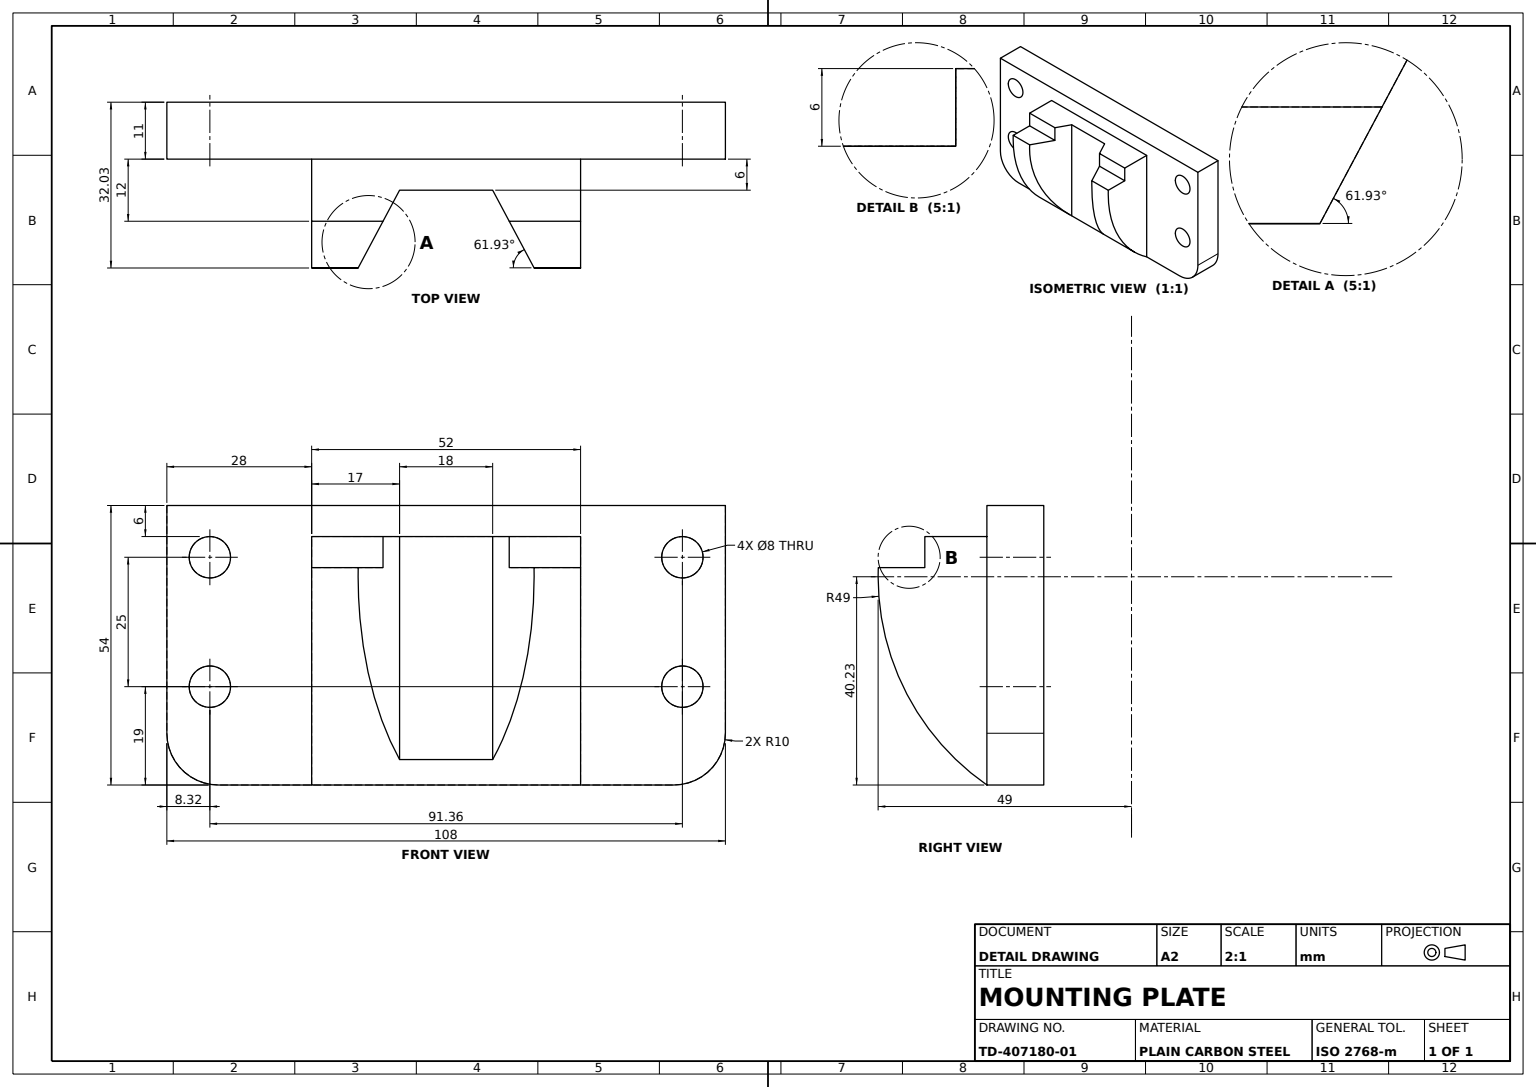
from build123d import *

# Parameters (mm, degrees)
BASE_PLATE_SKETCH_R   = 4
BASE_PLATE_DEPTH      = 11
GUIDE_BLOCK_DEPTH     = 26
CENTRE_SLOT_CUT_DEPTH = 26


with BuildPart() as part:
    # Base Plate Sketch → Base Plate (new body)
    with BuildSketch(Plane.XY):
        with BuildLine():
            Line((-54, 27), (54, 27))
            Line((54, 27), (54, -17))
            ThreePointArc((54, -17), (51.071067812, -24.071067812), (44, -27))
            Line((44, -27), (-44, -27))
            ThreePointArc((-44, -27), (-51.071067812, -24.071067812), (-54, -17))
            Line((-54, -17), (-54, 27))
        make_face()
        with Locations((-45.682264333, 17)):
            Circle(BASE_PLATE_SKETCH_R, mode=Mode.SUBTRACT)
        with Locations((-45.682264333, -8)):
            Circle(BASE_PLATE_SKETCH_R, mode=Mode.SUBTRACT)
        with Locations(Location((45.682264333, -8, 0), (0, 0, 180))):
            Circle(BASE_PLATE_SKETCH_R, mode=Mode.SUBTRACT)
        with Locations(Location((45.682264333, 17, 0), (0, 0, 180))):
            Circle(BASE_PLATE_SKETCH_R, mode=Mode.SUBTRACT)
    extrude(amount=BASE_PLATE_DEPTH)

    # Guide Block Profile → Guide Block (add, symmetric)
    with BuildSketch(Plane(origin=(0, 0, 0), x_dir=(0, 0, -1), z_dir=(1, 0, 0))):
        with BuildLine():
            Line((-11, 21), (-23, 21))
            Line((-23, 21), (-23, 15))
            Line((-23, 15), (-32, 15))
            ThreePointArc((-32, 15), (-26.8587637, -8.67938185), (-11, -27))
            Line((-11, -27), (-11, 21))
        make_face()
    extrude(amount=GUIDE_BLOCK_DEPTH, both=True)

    # Centre Slot Sketch → Centre Slot Cut (cut, symmetric)
    with BuildSketch(Plane(origin=(0, 0, 0), x_dir=(1, 0, 0), z_dir=(0, 1, 0))):
        Polygon((-9, -17), (-23.387504735, -43.976571377), (23.387504735, -43.976571377), (9, -17), align=None)
    extrude(amount=CENTRE_SLOT_CUT_DEPTH, both=True, mode=Mode.SUBTRACT)


solid = part.part
